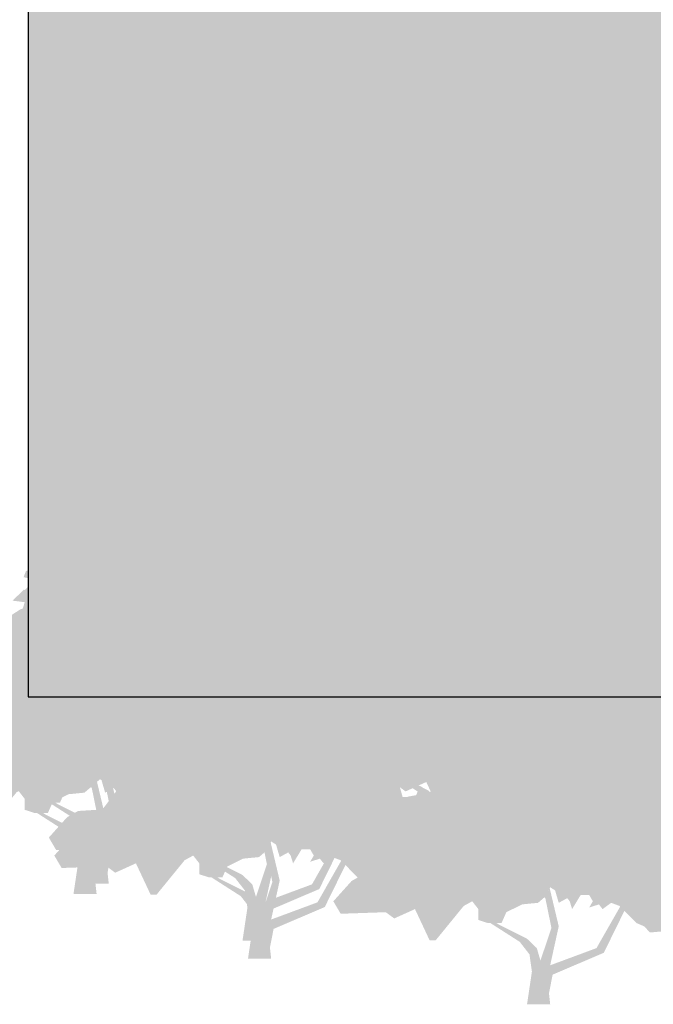
# Model space of a CAD drawing. Units: feet. Extents: x 2368 to 3224, y 836 to 1229.
# Tile 2 of 9: x 2395 to 2413, y 844 to 873. Entities that reach past the tile are written whole.
import ezdxf

# ---------------------------------------------------------------- set-up
doc = ezdxf.new("R2010")
doc.units = ezdxf.units.FT
for name, color, linetype, lineweight in [('A-ELEV', 7, 'Continuous', 25), ('A-ELEV-PATT', 8, 'Continuous', 13), ('L-PLNT', 3, 'Continuous', 13)]:
    doc.layers.add(name, color=color, linetype=linetype, lineweight=lineweight)

msp = doc.modelspace()

# ---------------------------------------------------------------- hatches: boundary and pattern name
at = {"layer": 'A-ELEV-PATT'}
h = msp.add_hatch(color=256, dxfattribs=at)
h.dxf.hatch_style = 1
h.paths.add_polyline_path([(2443.042, 973.51), (2394.909, 973.51), (2394.909, 853.51), (2443.042, 853.51)])
h.paths.add_polyline_path([(2422.205, 920.108), (2422.205, 905.784), (2416.403, 905.784), (2416.403, 920.108)], flags=16)
h.paths.add_polyline_path([(2449.299, 970.694), (2443.042, 973.51), (2443.042, 853.51), (2449.299, 853.51)])
h.paths.add_polyline_path([(2510.022, 987.861), (2368.302, 987.861), (2394.909, 973.51), (2443.042, 973.51), (2510.022, 973.51)])
h.paths.add_polyline_path([(2510.022, 973.51), (2443.042, 973.51), (2449.299, 970.694), (2510.022, 970.694)])
at = {"layer": 'L-PLNT'}
h = msp.add_hatch(color=256, dxfattribs=at)
h.dxf.hatch_style = 1
h.paths.add_polyline_path([(2411.665, 856.088), (2411.09, 856.687), (2410.371, 856.917), (2410.694, 857.424), (2410.407, 858.3), (2410.227, 858.3), (2409.868, 859.083), (2409.652, 859.037), (2409.4, 859.037), (2409.221, 859.406), (2409.328, 859.913), (2409.616, 859.913), (2409.077, 860.558), (2409.004, 861.069), (2408.717, 861.387), (2408.466, 861.111), (2408.322, 861.203), (2408.286, 861.433), (2408.106, 861.525), (2407.855, 861.295), (2407.567, 861.341), (2407.352, 860.926), (2407.352, 860.558), (2407.639, 860.419), (2407.423, 860.281), (2407.208, 860.466), (2406.597, 859.867), (2406.597, 859.728), (2406.345, 859.59), (2406.417, 859.452), (2406.597, 859.175), (2406.273, 858.945), (2405.95, 859.175), (2405.77, 859.129), (2405.698, 858.945), (2405.95, 858.899), (2405.986, 858.53), (2405.705, 858.576), (2405.375, 858.254), (2405.734, 858.208), (2405.59, 857.747), (2405.267, 857.701), (2404.907, 857.47), (2404.476, 857.24), (2404.44, 857.424), (2404.116, 856.733), (2404.692, 856.871), (2405.051, 856.641), (2404.943, 856.088), (2404.296, 855.857), (2404.009, 856.042), (2403.901, 855.765), (2403.649, 855.719), (2403.434, 855.443), (2403.182, 855.12), (2403.505, 854.844), (2403.721, 854.982), (2403.477, 854.581), (2403.654, 854.602), (2403.629, 854.239), (2403.038, 853.461), (2402.319, 853.415), (2401.996, 853.231), (2401.457, 852.632), (2401.672, 852.263), (2403.002, 852.309), (2403.254, 852.125), (2403.865, 852.401), (2404.296, 851.48), (2404.476, 851.48), (2405.303, 852.493), (2405.554, 852.632), (2405.734, 852.401), (2405.734, 852.079), (2406.022, 851.987), (2406.417, 851.987), (2406.561, 852.309), (2407.028, 852.54), (2407.495, 852.586), (2407.711, 852.77), (2407.747, 852.816), (2407.855, 853.046), (2407.999, 852.954), (2408.106, 852.586), (2408.358, 852.724), (2408.43, 852.632), (2408.502, 852.401), (2408.753, 852.816), (2409.005, 852.816), (2409.113, 852.632), (2409.005, 852.447), (2409.293, 852.54), (2409.4, 852.401), (2409.652, 852.586), (2409.904, 852.493), (2410.407, 851.987), (2410.622, 851.894), (2410.802, 851.71), (2412.312, 851.848), (2412.599, 851.572), (2412.815, 851.664), (2412.24, 852.401), (2412.204, 852.678), (2412.384, 852.954), (2412.06, 853.83), (2411.881, 853.83), (2411.521, 855.12), (2411.162, 855.166), (2411.377, 855.351)])
h = msp.add_hatch(color=256, dxfattribs=at)
h.dxf.hatch_style = 1
h.paths.add_polyline_path([(2411.214, 855.304), (2410.639, 855.904), (2409.92, 856.134), (2410.243, 856.641), (2409.956, 857.516), (2409.776, 857.516), (2409.417, 858.3), (2409.201, 858.254), (2408.949, 858.254), (2408.77, 858.622), (2408.878, 859.129), (2409.165, 859.129), (2408.626, 859.774), (2408.553, 860.286), (2408.266, 860.604), (2408.015, 860.327), (2407.871, 860.42), (2407.835, 860.65), (2407.655, 860.742), (2407.404, 860.512), (2407.116, 860.558), (2406.901, 860.143), (2406.901, 859.774), (2407.188, 859.636), (2406.972, 859.498), (2406.757, 859.682), (2406.146, 859.083), (2406.146, 858.945), (2405.894, 858.807), (2405.966, 858.668), (2406.146, 858.392), (2405.822, 858.162), (2405.499, 858.392), (2405.319, 858.346), (2405.247, 858.162), (2405.499, 858.115), (2405.535, 857.747), (2405.254, 857.793), (2404.924, 857.47), (2405.283, 857.424), (2405.139, 856.963), (2404.816, 856.917), (2404.456, 856.687), (2404.025, 856.456), (2403.989, 856.641), (2403.666, 855.95), (2404.241, 856.088), (2404.6, 855.857), (2404.492, 855.304), (2403.845, 855.074), (2403.558, 855.258), (2403.45, 854.982), (2403.198, 854.936), (2402.983, 854.659), (2402.731, 854.337), (2403.054, 854.06), (2403.27, 854.199), (2403.026, 853.798), (2403.203, 853.818), (2403.178, 853.456), (2402.587, 852.678), (2401.868, 852.632), (2401.545, 852.447), (2401.006, 851.848), (2401.221, 851.48), (2402.551, 851.526), (2402.803, 851.341), (2403.414, 851.618), (2403.845, 850.696), (2404.025, 850.696), (2404.852, 851.71), (2405.103, 851.848), (2405.283, 851.618), (2405.283, 851.295), (2405.571, 851.203), (2405.966, 851.203), (2406.11, 851.526), (2406.577, 851.756), (2407.044, 851.802), (2407.26, 851.987), (2407.296, 852.033), (2407.404, 852.263), (2407.548, 852.171), (2407.655, 851.802), (2407.907, 851.941), (2407.979, 851.848), (2408.051, 851.618), (2408.302, 852.033), (2408.554, 852.033), (2408.662, 851.848), (2408.554, 851.664), (2408.842, 851.756), (2408.949, 851.618), (2409.201, 851.802), (2409.453, 851.71), (2409.956, 851.203), (2410.172, 851.111), (2410.351, 850.927), (2411.861, 851.065), (2412.149, 850.788), (2412.364, 850.881), (2411.789, 851.618), (2411.753, 851.894), (2411.933, 852.171), (2411.609, 853.046), (2411.43, 853.046), (2411.07, 854.337), (2410.711, 854.383), (2410.926, 854.567)])
h = msp.add_hatch(color=256, dxfattribs=at)
h.dxf.hatch_style = 1
h.paths.add_polyline_path([(2414.456, 854.681), (2413.881, 855.281), (2413.162, 855.511), (2413.485, 856.018), (2413.198, 856.893), (2413.018, 856.893), (2412.659, 857.677), (2412.443, 857.631), (2412.191, 857.631), (2412.012, 857.999), (2412.12, 858.506), (2412.407, 858.506), (2411.868, 859.151), (2411.795, 859.663), (2411.509, 859.981), (2411.257, 859.704), (2411.113, 859.797), (2411.077, 860.027), (2410.897, 860.119), (2410.646, 859.889), (2410.358, 859.935), (2410.143, 859.52), (2410.143, 859.151), (2410.43, 859.013), (2410.214, 858.875), (2409.999, 859.059), (2409.388, 858.46), (2409.388, 858.322), (2409.136, 858.184), (2409.208, 858.045), (2409.388, 857.769), (2409.064, 857.539), (2408.741, 857.769), (2408.561, 857.723), (2408.489, 857.539), (2408.741, 857.492), (2408.777, 857.124), (2408.496, 857.17), (2408.166, 856.847), (2408.525, 856.801), (2408.381, 856.34), (2408.058, 856.294), (2407.698, 856.064), (2407.267, 855.834), (2407.231, 856.018), (2406.908, 855.327), (2407.483, 855.465), (2407.842, 855.234), (2407.734, 854.681), (2407.087, 854.451), (2406.8, 854.635), (2406.692, 854.359), (2406.44, 854.313), (2406.225, 854.036), (2405.973, 853.714), (2406.297, 853.437), (2406.512, 853.576), (2406.268, 853.175), (2406.445, 853.195), (2406.42, 852.833), (2405.829, 852.055), (2405.11, 852.009), (2404.787, 851.824), (2404.248, 851.225), (2404.463, 850.857), (2405.793, 850.903), (2406.045, 850.718), (2406.656, 850.995), (2407.087, 850.073), (2407.267, 850.073), (2408.094, 851.087), (2408.345, 851.225), (2408.525, 850.995), (2408.525, 850.672), (2408.813, 850.58), (2409.208, 850.58), (2409.352, 850.903), (2409.819, 851.133), (2410.286, 851.179), (2410.502, 851.364), (2410.538, 851.41), (2410.646, 851.64), (2410.79, 851.548), (2410.897, 851.179), (2411.149, 851.318), (2411.221, 851.225), (2411.293, 850.995), (2411.544, 851.41), (2411.796, 851.41), (2411.904, 851.225), (2411.796, 851.041), (2412.084, 851.133), (2412.191, 850.995), (2412.443, 851.179), (2412.695, 851.087), (2413.198, 850.58), (2413.414, 850.488), (2413.593, 850.304), (2415.103, 850.442), (2415.391, 850.165), (2415.606, 850.258), (2415.031, 850.995), (2414.995, 851.271), (2415.175, 851.548), (2414.851, 852.423), (2414.672, 852.423), (2414.312, 853.714), (2413.953, 853.76), (2414.168, 853.944)])
h = msp.add_hatch(color=256, dxfattribs=at)
h.dxf.hatch_style = 1
h.paths.add_polyline_path([(2421.127, 854.737), (2420.552, 855.336), (2419.833, 855.567), (2420.157, 856.074), (2419.869, 856.949), (2419.689, 856.949), (2419.33, 857.732), (2419.114, 857.686), (2418.862, 857.686), (2418.683, 858.055), (2418.791, 858.562), (2419.078, 858.562), (2418.539, 859.207), (2418.466, 859.718), (2418.18, 860.037), (2417.928, 859.76), (2417.784, 859.852), (2417.748, 860.083), (2417.568, 860.175), (2417.317, 859.944), (2417.029, 859.99), (2416.814, 859.576), (2416.814, 859.207), (2417.101, 859.069), (2416.886, 858.931), (2416.67, 859.115), (2416.059, 858.516), (2416.059, 858.378), (2415.807, 858.239), (2415.879, 858.101), (2416.059, 857.825), (2415.735, 857.594), (2415.412, 857.825), (2415.232, 857.779), (2415.16, 857.594), (2415.412, 857.548), (2415.448, 857.179), (2415.167, 857.226), (2414.837, 856.903), (2415.196, 856.857), (2415.052, 856.396), (2414.729, 856.35), (2414.369, 856.12), (2413.938, 855.889), (2413.902, 856.074), (2413.579, 855.382), (2414.154, 855.521), (2414.513, 855.29), (2414.405, 854.737), (2413.758, 854.507), (2413.471, 854.691), (2413.363, 854.415), (2413.111, 854.369), (2412.896, 854.092), (2412.644, 853.769), (2412.968, 853.493), (2413.183, 853.631), (2412.939, 853.23), (2413.117, 853.251), (2413.091, 852.888), (2412.5, 852.111), (2411.781, 852.064), (2411.458, 851.88), (2410.919, 851.281), (2411.134, 850.912), (2412.464, 850.958), (2412.716, 850.774), (2413.327, 851.051), (2413.758, 850.129), (2413.938, 850.129), (2414.765, 851.143), (2415.016, 851.281), (2415.196, 851.051), (2415.196, 850.728), (2415.484, 850.636), (2415.879, 850.636), (2416.023, 850.958), (2416.49, 851.189), (2416.957, 851.235), (2417.173, 851.419), (2417.209, 851.465), (2417.317, 851.696), (2417.461, 851.604), (2417.568, 851.235), (2417.82, 851.373), (2417.892, 851.281), (2417.964, 851.051), (2418.215, 851.465), (2418.467, 851.465), (2418.575, 851.281), (2418.467, 851.097), (2418.755, 851.189), (2418.862, 851.051), (2419.114, 851.235), (2419.366, 851.143), (2419.869, 850.636), (2420.085, 850.544), (2420.264, 850.359), (2421.774, 850.498), (2422.062, 850.221), (2422.277, 850.313), (2421.702, 851.051), (2421.666, 851.327), (2421.846, 851.604), (2421.522, 852.479), (2421.343, 852.479), (2420.983, 853.769), (2420.624, 853.816), (2420.839, 854)])
h = msp.add_hatch(color=256, dxfattribs=at)
h.dxf.hatch_style = 1
h.paths.add_polyline_path([(2401.097, 854.492), (2400.522, 855.091), (2399.803, 855.321), (2400.126, 855.828), (2399.839, 856.704), (2399.659, 856.704), (2399.3, 857.487), (2399.084, 857.441), (2398.832, 857.441), (2398.653, 857.809), (2398.76, 858.316), (2399.048, 858.316), (2398.509, 858.962), (2398.436, 859.473), (2398.149, 859.791), (2397.898, 859.514), (2397.754, 859.607), (2397.718, 859.837), (2397.538, 859.929), (2397.287, 859.699), (2396.999, 859.745), (2396.783, 859.33), (2396.783, 858.962), (2397.071, 858.823), (2396.855, 858.685), (2396.64, 858.869), (2396.029, 858.27), (2396.029, 858.132), (2395.777, 857.994), (2395.849, 857.856), (2396.029, 857.579), (2395.705, 857.349), (2395.382, 857.579), (2395.202, 857.533), (2395.13, 857.349), (2395.382, 857.303), (2395.418, 856.934), (2395.136, 856.98), (2394.806, 856.657), (2395.166, 856.611), (2395.022, 856.151), (2394.699, 856.104), (2394.339, 855.874), (2393.908, 855.644), (2393.872, 855.828), (2393.548, 855.137), (2394.124, 855.275), (2394.483, 855.045), (2394.375, 854.492), (2393.728, 854.261), (2393.441, 854.446), (2393.333, 854.169), (2393.081, 854.123), (2392.865, 853.846), (2392.614, 853.524), (2392.937, 853.247), (2393.153, 853.386), (2392.909, 852.985), (2393.086, 853.006), (2393.061, 852.643), (2392.47, 851.865), (2391.751, 851.819), (2391.428, 851.635), (2390.888, 851.035), (2391.104, 850.667), (2392.434, 850.713), (2392.686, 850.529), (2393.297, 850.805), (2393.728, 849.883), (2393.908, 849.883), (2394.735, 850.897), (2394.986, 851.035), (2395.166, 850.805), (2395.166, 850.483), (2395.453, 850.39), (2395.849, 850.39), (2395.993, 850.713), (2396.46, 850.943), (2396.927, 850.989), (2397.143, 851.174), (2397.179, 851.22), (2397.287, 851.45), (2397.43, 851.358), (2397.538, 850.989), (2397.79, 851.128), (2397.862, 851.035), (2397.934, 850.805), (2398.185, 851.22), (2398.437, 851.22), (2398.545, 851.035), (2398.437, 850.851), (2398.724, 850.943), (2398.832, 850.805), (2399.084, 850.989), (2399.336, 850.897), (2399.839, 850.39), (2400.054, 850.298), (2400.234, 850.114), (2401.744, 850.252), (2402.031, 849.976), (2402.247, 850.068), (2401.672, 850.805), (2401.636, 851.082), (2401.816, 851.358), (2401.492, 852.234), (2401.312, 852.234), (2400.953, 853.524), (2400.594, 853.57), (2400.809, 853.754)])
h = msp.add_hatch(color=256, dxfattribs=at)
h.dxf.hatch_style = 1
h.paths.add_polyline_path([(2400.74, 854.183), (2400.164, 854.782), (2399.446, 855.013), (2399.769, 855.519), (2399.482, 856.395), (2399.302, 856.395), (2398.942, 857.178), (2398.727, 857.132), (2398.475, 857.132), (2398.295, 857.501), (2398.403, 858.008), (2398.691, 858.008), (2398.152, 858.653), (2398.079, 859.164), (2397.792, 859.482), (2397.54, 859.206), (2397.397, 859.298), (2397.361, 859.529), (2397.181, 859.621), (2396.929, 859.39), (2396.642, 859.436), (2396.426, 859.022), (2396.426, 858.653), (2396.714, 858.515), (2396.498, 858.377), (2396.282, 858.561), (2395.671, 857.962), (2395.671, 857.824), (2395.42, 857.685), (2395.492, 857.547), (2395.671, 857.271), (2395.348, 857.04), (2395.024, 857.271), (2394.845, 857.224), (2394.773, 857.04), (2395.024, 856.994), (2395.06, 856.625), (2394.779, 856.672), (2394.449, 856.349), (2394.809, 856.303), (2394.665, 855.842), (2394.341, 855.796), (2393.982, 855.566), (2393.551, 855.335), (2393.515, 855.519), (2393.191, 854.828), (2393.766, 854.966), (2394.126, 854.736), (2394.018, 854.183), (2393.371, 853.953), (2393.083, 854.137), (2392.975, 853.861), (2392.724, 853.814), (2392.508, 853.538), (2392.257, 853.215), (2392.58, 852.939), (2392.796, 853.077), (2392.552, 852.676), (2392.729, 852.697), (2392.703, 852.334), (2392.113, 851.556), (2391.394, 851.51), (2391.07, 851.326), (2390.531, 850.727), (2390.747, 850.358), (2392.077, 850.404), (2392.328, 850.22), (2392.94, 850.497), (2393.371, 849.575), (2393.551, 849.575), (2394.377, 850.589), (2394.629, 850.727), (2394.809, 850.497), (2394.809, 850.174), (2395.096, 850.082), (2395.492, 850.082), (2395.635, 850.404), (2396.103, 850.635), (2396.57, 850.681), (2396.786, 850.865), (2396.822, 850.911), (2396.929, 851.142), (2397.073, 851.05), (2397.181, 850.681), (2397.433, 850.819), (2397.505, 850.727), (2397.576, 850.497), (2397.828, 850.911), (2398.08, 850.911), (2398.187, 850.727), (2398.08, 850.543), (2398.367, 850.635), (2398.475, 850.497), (2398.727, 850.681), (2398.978, 850.589), (2399.482, 850.082), (2399.697, 849.99), (2399.877, 849.805), (2401.387, 849.944), (2401.674, 849.667), (2401.89, 849.759), (2401.315, 850.497), (2401.279, 850.773), (2401.458, 851.05), (2401.135, 851.925), (2400.955, 851.925), (2400.596, 853.215), (2400.236, 853.261), (2400.452, 853.446)])
h = msp.add_hatch(color=256, dxfattribs=at)
h.dxf.hatch_style = 1
h.paths.add_polyline_path([(2422.561, 854.308), (2421.986, 854.907), (2421.267, 855.137), (2421.591, 855.644), (2421.303, 856.52), (2421.123, 856.52), (2420.764, 857.303), (2420.548, 857.257), (2420.297, 857.257), (2420.117, 857.626), (2420.225, 858.132), (2420.512, 858.132), (2419.973, 858.778), (2419.901, 859.289), (2419.614, 859.607), (2419.362, 859.331), (2419.218, 859.423), (2419.182, 859.653), (2419.003, 859.745), (2418.751, 859.515), (2418.463, 859.561), (2418.248, 859.146), (2418.248, 858.778), (2418.535, 858.639), (2418.32, 858.501), (2418.104, 858.685), (2417.493, 858.086), (2417.493, 857.948), (2417.241, 857.81), (2417.313, 857.672), (2417.493, 857.395), (2417.169, 857.165), (2416.846, 857.395), (2416.666, 857.349), (2416.594, 857.165), (2416.846, 857.119), (2416.882, 856.75), (2416.601, 856.796), (2416.271, 856.474), (2416.63, 856.427), (2416.486, 855.967), (2416.163, 855.921), (2415.804, 855.69), (2415.372, 855.46), (2415.336, 855.644), (2415.013, 854.953), (2415.588, 855.091), (2415.947, 854.861), (2415.839, 854.308), (2415.192, 854.077), (2414.905, 854.262), (2414.797, 853.985), (2414.545, 853.939), (2414.33, 853.663), (2414.078, 853.34), (2414.402, 853.063), (2414.617, 853.202), (2414.374, 852.801), (2414.551, 852.822), (2414.525, 852.459), (2413.934, 851.681), (2413.215, 851.635), (2412.892, 851.451), (2412.353, 850.852), (2412.568, 850.483), (2413.898, 850.529), (2414.15, 850.345), (2414.761, 850.621), (2415.192, 849.7), (2415.372, 849.7), (2416.199, 850.713), (2416.451, 850.852), (2416.63, 850.621), (2416.63, 850.299), (2416.918, 850.206), (2417.313, 850.206), (2417.457, 850.529), (2417.924, 850.759), (2418.392, 850.806), (2418.607, 850.99), (2418.643, 851.036), (2418.751, 851.266), (2418.895, 851.174), (2419.003, 850.806), (2419.254, 850.944), (2419.326, 850.852), (2419.398, 850.621), (2419.65, 851.036), (2419.901, 851.036), (2420.009, 850.852), (2419.901, 850.667), (2420.189, 850.759), (2420.297, 850.621), (2420.548, 850.806), (2420.8, 850.713), (2421.303, 850.206), (2421.519, 850.114), (2421.698, 849.93), (2423.208, 850.068), (2423.496, 849.792), (2423.711, 849.884), (2423.136, 850.621), (2423.1, 850.898), (2423.28, 851.174), (2422.957, 852.05), (2422.777, 852.05), (2422.417, 853.34), (2422.058, 853.386), (2422.274, 853.57)])
h = msp.add_hatch(color=256, dxfattribs=at)
h.dxf.hatch_style = 1
h.paths.add_polyline_path([(2405.727, 852.813), (2405.152, 853.412), (2404.433, 853.642), (2404.757, 854.149), (2404.469, 855.024), (2404.29, 855.024), (2403.93, 855.808), (2403.714, 855.762), (2403.463, 855.762), (2403.283, 856.13), (2403.391, 856.637), (2403.679, 856.637), (2403.139, 857.282), (2403.067, 857.794), (2402.78, 858.112), (2402.528, 857.835), (2402.384, 857.928), (2402.349, 858.158), (2402.169, 858.25), (2401.917, 858.02), (2401.63, 858.066), (2401.414, 857.651), (2401.414, 857.282), (2401.702, 857.144), (2401.486, 857.006), (2401.27, 857.19), (2400.659, 856.591), (2400.659, 856.453), (2400.408, 856.315), (2400.479, 856.177), (2400.659, 855.9), (2400.336, 855.67), (2400.012, 855.9), (2399.832, 855.854), (2399.761, 855.67), (2400.012, 855.624), (2400.048, 855.255), (2399.767, 855.301), (2399.437, 854.978), (2399.796, 854.932), (2399.653, 854.471), (2399.329, 854.425), (2398.97, 854.195), (2398.538, 853.965), (2398.502, 854.149), (2398.179, 853.458), (2398.754, 853.596), (2399.114, 853.366), (2399.006, 852.813), (2398.359, 852.582), (2398.071, 852.766), (2397.963, 852.49), (2397.712, 852.444), (2397.496, 852.167), (2397.244, 851.845), (2397.568, 851.568), (2397.784, 851.707), (2397.54, 851.306), (2397.717, 851.327), (2397.691, 850.964), (2397.101, 850.186), (2396.382, 850.14), (2396.058, 849.956), (2395.519, 849.356), (2395.735, 848.988), (2397.065, 849.034), (2397.316, 848.85), (2397.927, 849.126), (2398.359, 848.204), (2398.538, 848.204), (2399.365, 849.218), (2399.617, 849.356), (2399.796, 849.126), (2399.796, 848.803), (2400.084, 848.711), (2400.479, 848.711), (2400.623, 849.034), (2401.09, 849.264), (2401.558, 849.31), (2401.773, 849.495), (2401.809, 849.541), (2401.917, 849.771), (2402.061, 849.679), (2402.169, 849.31), (2402.42, 849.449), (2402.492, 849.356), (2402.564, 849.126), (2402.816, 849.541), (2403.067, 849.541), (2403.175, 849.356), (2403.067, 849.172), (2403.355, 849.264), (2403.463, 849.126), (2403.714, 849.31), (2403.966, 849.218), (2404.469, 848.711), (2404.685, 848.619), (2404.865, 848.435), (2406.374, 848.573), (2406.662, 848.297), (2406.878, 848.389), (2406.302, 849.126), (2406.267, 849.403), (2406.446, 849.679), (2406.123, 850.555), (2405.943, 850.555), (2405.584, 851.845), (2405.224, 851.891), (2405.44, 852.075)])
h = msp.add_hatch(color=256, dxfattribs=at)
h.dxf.hatch_style = 1
h.paths.add_polyline_path([(2405.889, 852.281), (2405.314, 852.88), (2404.595, 853.111), (2404.919, 853.618), (2404.631, 854.493), (2404.452, 854.493), (2404.092, 855.277), (2403.876, 855.231), (2403.625, 855.231), (2403.445, 855.599), (2403.553, 856.106), (2403.84, 856.106), (2403.301, 856.751), (2403.229, 857.263), (2402.942, 857.581), (2402.69, 857.304), (2402.546, 857.396), (2402.51, 857.627), (2402.331, 857.719), (2402.079, 857.489), (2401.792, 857.535), (2401.576, 857.12), (2401.576, 856.751), (2401.863, 856.613), (2401.648, 856.475), (2401.432, 856.659), (2400.821, 856.06), (2400.821, 855.922), (2400.569, 855.784), (2400.641, 855.645), (2400.821, 855.369), (2400.498, 855.138), (2400.174, 855.369), (2399.994, 855.323), (2399.922, 855.138), (2400.174, 855.092), (2400.21, 854.724), (2399.929, 854.77), (2399.599, 854.447), (2399.958, 854.401), (2399.815, 853.94), (2399.491, 853.894), (2399.132, 853.664), (2398.7, 853.433), (2398.664, 853.618), (2398.341, 852.927), (2398.916, 853.065), (2399.275, 852.834), (2399.168, 852.281), (2398.521, 852.051), (2398.233, 852.235), (2398.125, 851.959), (2397.874, 851.913), (2397.658, 851.636), (2397.406, 851.314), (2397.73, 851.037), (2397.946, 851.175), (2397.702, 850.775), (2397.879, 850.795), (2397.853, 850.433), (2397.263, 849.655), (2396.544, 849.609), (2396.22, 849.424), (2395.681, 848.825), (2395.897, 848.457), (2397.227, 848.503), (2397.478, 848.318), (2398.089, 848.595), (2398.521, 847.673), (2398.7, 847.673), (2399.527, 848.687), (2399.779, 848.825), (2399.958, 848.595), (2399.958, 848.272), (2400.246, 848.18), (2400.641, 848.18), (2400.785, 848.503), (2401.252, 848.733), (2401.72, 848.779), (2401.935, 848.964), (2401.971, 849.01), (2402.079, 849.24), (2402.223, 849.148), (2402.331, 848.779), (2402.582, 848.917), (2402.654, 848.825), (2402.726, 848.595), (2402.978, 849.01), (2403.229, 849.01), (2403.337, 848.825), (2403.229, 848.641), (2403.517, 848.733), (2403.625, 848.595), (2403.876, 848.779), (2404.128, 848.687), (2404.631, 848.18), (2404.847, 848.088), (2405.027, 847.904), (2406.536, 848.042), (2406.824, 847.765), (2407.04, 847.858), (2406.464, 848.595), (2406.428, 848.871), (2406.608, 849.148), (2406.285, 850.023), (2406.105, 850.023), (2405.746, 851.314), (2405.386, 851.36), (2405.602, 851.544)])
h = msp.add_hatch(color=256, dxfattribs=at)
h.dxf.hatch_style = 1
h.paths.add_polyline_path([(2419.444, 852.439), (2418.869, 853.038), (2418.15, 853.268), (2418.473, 853.775), (2418.186, 854.651), (2418.006, 854.651), (2417.647, 855.434), (2417.431, 855.388), (2417.179, 855.388), (2417, 855.757), (2417.107, 856.264), (2417.395, 856.264), (2416.856, 856.909), (2416.783, 857.42), (2416.496, 857.738), (2416.245, 857.462), (2416.101, 857.554), (2416.065, 857.784), (2415.885, 857.876), (2415.634, 857.646), (2415.346, 857.692), (2415.13, 857.277), (2415.13, 856.909), (2415.418, 856.77), (2415.202, 856.632), (2414.987, 856.817), (2414.376, 856.217), (2414.376, 856.079), (2414.124, 855.941), (2414.196, 855.803), (2414.376, 855.526), (2414.052, 855.296), (2413.729, 855.526), (2413.549, 855.48), (2413.477, 855.296), (2413.729, 855.25), (2413.764, 854.881), (2413.483, 854.927), (2413.153, 854.605), (2413.513, 854.559), (2413.369, 854.098), (2413.046, 854.052), (2412.686, 853.821), (2412.255, 853.591), (2412.219, 853.775), (2411.895, 853.084), (2412.47, 853.222), (2412.83, 852.992), (2412.722, 852.439), (2412.075, 852.208), (2411.788, 852.393), (2411.68, 852.116), (2411.428, 852.07), (2411.212, 851.794), (2410.961, 851.471), (2411.284, 851.195), (2411.5, 851.333), (2411.256, 850.932), (2411.433, 850.953), (2411.408, 850.59), (2410.817, 849.812), (2410.098, 849.766), (2409.775, 849.582), (2409.235, 848.983), (2409.451, 848.614), (2410.781, 848.66), (2411.033, 848.476), (2411.644, 848.752), (2412.075, 847.831), (2412.255, 847.831), (2413.082, 848.844), (2413.333, 848.983), (2413.513, 848.752), (2413.513, 848.43), (2413.8, 848.338), (2414.196, 848.338), (2414.34, 848.66), (2414.807, 848.89), (2415.274, 848.937), (2415.49, 849.121), (2415.526, 849.167), (2415.634, 849.397), (2415.777, 849.305), (2415.885, 848.937), (2416.137, 849.075), (2416.209, 848.983), (2416.281, 848.752), (2416.532, 849.167), (2416.784, 849.167), (2416.892, 848.983), (2416.784, 848.798), (2417.071, 848.89), (2417.179, 848.752), (2417.431, 848.937), (2417.682, 848.844), (2418.186, 848.338), (2418.401, 848.245), (2418.581, 848.061), (2420.091, 848.199), (2420.378, 847.923), (2420.594, 848.015), (2420.019, 848.752), (2419.983, 849.029), (2420.163, 849.305), (2419.839, 850.181), (2419.659, 850.181), (2419.3, 851.471), (2418.941, 851.517), (2419.156, 851.701)])
h = msp.add_hatch(color=256, dxfattribs=at)
h.dxf.hatch_style = 1
h.paths.add_polyline_path([(2414.123, 850.931), (2413.547, 851.53), (2412.829, 851.76), (2413.152, 852.267), (2412.865, 853.143), (2412.685, 853.143), (2412.325, 853.926), (2412.11, 853.88), (2411.858, 853.88), (2411.678, 854.249), (2411.786, 854.756), (2412.074, 854.756), (2411.535, 855.401), (2411.462, 855.912), (2411.175, 856.23), (2410.924, 855.954), (2410.78, 856.046), (2410.744, 856.276), (2410.564, 856.368), (2410.312, 856.138), (2410.025, 856.184), (2409.809, 855.769), (2409.809, 855.401), (2410.097, 855.262), (2409.881, 855.124), (2409.665, 855.309), (2409.054, 854.709), (2409.054, 854.571), (2408.803, 854.433), (2408.875, 854.295), (2409.054, 854.018), (2408.731, 853.788), (2408.407, 854.018), (2408.228, 853.972), (2408.156, 853.788), (2408.407, 853.742), (2408.443, 853.373), (2408.162, 853.419), (2407.832, 853.097), (2408.192, 853.051), (2408.048, 852.59), (2407.724, 852.544), (2407.365, 852.313), (2406.934, 852.083), (2406.898, 852.267), (2406.574, 851.576), (2407.149, 851.714), (2407.509, 851.484), (2407.401, 850.931), (2406.754, 850.7), (2406.466, 850.885), (2406.359, 850.608), (2406.107, 850.562), (2405.891, 850.286), (2405.64, 849.963), (2405.963, 849.687), (2406.179, 849.825), (2405.935, 849.424), (2406.112, 849.445), (2406.086, 849.082), (2405.496, 848.304), (2404.777, 848.258), (2404.453, 848.074), (2403.914, 847.475), (2404.13, 847.106), (2405.46, 847.152), (2405.711, 846.968), (2406.323, 847.244), (2406.754, 846.323), (2406.934, 846.323), (2407.76, 847.336), (2408.012, 847.475), (2408.192, 847.244), (2408.192, 846.922), (2408.479, 846.83), (2408.875, 846.83), (2409.018, 847.152), (2409.486, 847.383), (2409.953, 847.429), (2410.169, 847.613), (2410.205, 847.659), (2410.312, 847.889), (2410.456, 847.797), (2410.564, 847.429), (2410.816, 847.567), (2410.888, 847.475), (2410.959, 847.244), (2411.211, 847.659), (2411.463, 847.659), (2411.571, 847.475), (2411.463, 847.29), (2411.75, 847.383), (2411.858, 847.244), (2412.11, 847.429), (2412.361, 847.336), (2412.865, 846.83), (2413.08, 846.737), (2413.26, 846.553), (2414.77, 846.691), (2415.057, 846.415), (2415.273, 846.507), (2414.698, 847.244), (2414.662, 847.521), (2414.841, 847.797), (2414.518, 848.673), (2414.338, 848.673), (2413.979, 849.963), (2413.619, 850.009), (2413.835, 850.193)])
h = msp.add_hatch(color=256, dxfattribs=at)
h.dxf.hatch_style = 1
h.paths.add_polyline_path([(2407.927, 850.466), (2409.436, 851.111), (2410.045, 852.351), (2409.92, 852.477), (2409.904, 852.447), (2409.221, 851.249), (2407.855, 850.742), (2408.106, 851.894), (2407.855, 852.954), (2407.84, 853.015), (2407.747, 852.816), (2407.711, 852.77), (2407.688, 852.751), (2407.711, 852.724), (2407.891, 851.848), (2407.567, 850.881), (2407.459, 851.249), (2407.172, 851.526), (2406.345, 851.94), (2406.274, 851.987), (2406.093, 851.987), (2406.956, 851.434), (2407.244, 851.065), (2407.316, 850.558), (2407.172, 849.59), (2407.855, 849.59), (2407.819, 849.913)])
h = msp.add_hatch(color=256, dxfattribs=at)
h.dxf.hatch_style = 1
h.paths.add_polyline_path([(2407.476, 849.683), (2408.985, 850.328), (2409.594, 851.567), (2409.469, 851.693), (2409.453, 851.664), (2408.77, 850.466), (2407.404, 849.959), (2407.655, 851.111), (2407.404, 852.171), (2407.389, 852.232), (2407.296, 852.033), (2407.26, 851.987), (2407.237, 851.967), (2407.26, 851.941), (2407.44, 851.065), (2407.116, 850.097), (2407.008, 850.466), (2406.721, 850.742), (2405.894, 851.157), (2405.823, 851.203), (2405.642, 851.203), (2406.505, 850.65), (2406.793, 850.282), (2406.865, 849.775), (2406.721, 848.807), (2407.404, 848.807), (2407.368, 849.13)])
h = msp.add_hatch(color=256, dxfattribs=at)
h.dxf.hatch_style = 1
h.paths.add_polyline_path([(2397.359, 848.87), (2398.868, 849.515), (2399.477, 850.755), (2399.352, 850.88), (2399.336, 850.851), (2398.653, 849.653), (2397.287, 849.146), (2397.538, 850.298), (2397.287, 851.358), (2397.272, 851.419), (2397.179, 851.22), (2397.143, 851.174), (2397.12, 851.154), (2397.143, 851.128), (2397.323, 850.252), (2396.999, 849.284), (2396.891, 849.653), (2396.604, 849.93), (2395.777, 850.344), (2395.706, 850.39), (2395.525, 850.39), (2396.388, 849.837), (2396.676, 849.469), (2396.747, 848.962), (2396.604, 847.994), (2397.287, 847.994), (2397.251, 848.317)])
h = msp.add_hatch(color=256, dxfattribs=at)
h.dxf.hatch_style = 1
h.paths.add_polyline_path([(2410.718, 849.06), (2412.227, 849.705), (2412.836, 850.944), (2412.711, 851.07), (2412.695, 851.041), (2412.012, 849.843), (2410.646, 849.336), (2410.897, 850.488), (2410.646, 851.548), (2410.631, 851.609), (2410.538, 851.41), (2410.502, 851.364), (2410.479, 851.344), (2410.502, 851.318), (2410.682, 850.442), (2410.358, 849.474), (2410.25, 849.843), (2409.963, 850.119), (2409.136, 850.534), (2409.065, 850.58), (2408.885, 850.58), (2409.747, 850.027), (2410.035, 849.659), (2410.107, 849.152), (2409.963, 848.184), (2410.646, 848.184), (2410.61, 848.507)])
h = msp.add_hatch(color=256, dxfattribs=at)
h.dxf.hatch_style = 1
h.paths.add_polyline_path([(2397.001, 848.561), (2398.511, 849.206), (2399.12, 850.446), (2398.995, 850.572), (2398.978, 850.543), (2398.295, 849.345), (2396.929, 848.838), (2397.181, 849.99), (2396.929, 851.05), (2396.915, 851.111), (2396.822, 850.911), (2396.786, 850.865), (2396.763, 850.846), (2396.786, 850.819), (2396.965, 849.944), (2396.642, 848.976), (2396.534, 849.345), (2396.246, 849.621), (2395.42, 850.036), (2395.349, 850.082), (2395.168, 850.082), (2396.031, 849.529), (2396.318, 849.16), (2396.39, 848.653), (2396.246, 847.686), (2396.929, 847.686), (2396.893, 848.008)])
h = msp.add_hatch(color=256, dxfattribs=at)
h.dxf.hatch_style = 1
h.paths.add_polyline_path([(2401.989, 847.191), (2403.499, 847.836), (2404.108, 849.076), (2403.983, 849.201), (2403.966, 849.172), (2403.283, 847.974), (2401.917, 847.467), (2402.169, 848.619), (2401.917, 849.679), (2401.903, 849.74), (2401.809, 849.541), (2401.773, 849.495), (2401.751, 849.475), (2401.773, 849.449), (2401.953, 848.573), (2401.63, 847.605), (2401.522, 847.974), (2401.234, 848.25), (2400.408, 848.665), (2400.337, 848.711), (2400.156, 848.711), (2401.019, 848.158), (2401.306, 847.79), (2401.378, 847.283), (2401.234, 846.315), (2401.917, 846.315), (2401.881, 846.638)])
h = msp.add_hatch(color=256, dxfattribs=at)
h.dxf.hatch_style = 1
h.paths.add_polyline_path([(2402.151, 846.659), (2403.661, 847.305), (2404.27, 848.544), (2404.145, 848.67), (2404.128, 848.641), (2403.445, 847.443), (2402.079, 846.936), (2402.331, 848.088), (2402.079, 849.148), (2402.065, 849.209), (2401.971, 849.01), (2401.935, 848.964), (2401.913, 848.944), (2401.935, 848.917), (2402.115, 848.042), (2401.792, 847.074), (2401.684, 847.443), (2401.396, 847.719), (2400.569, 848.134), (2400.499, 848.18), (2400.318, 848.18), (2401.181, 847.627), (2401.468, 847.259), (2401.54, 846.752), (2401.396, 845.784), (2402.079, 845.784), (2402.043, 846.107)])
h = msp.add_hatch(color=256, dxfattribs=at)
h.dxf.hatch_style = 1
h.paths.add_polyline_path([(2410.384, 845.309), (2411.894, 845.954), (2412.503, 847.194), (2412.378, 847.32), (2412.361, 847.29), (2411.678, 846.092), (2410.312, 845.585), (2410.564, 846.737), (2410.312, 847.797), (2410.298, 847.858), (2410.205, 847.659), (2410.169, 847.613), (2410.146, 847.593), (2410.169, 847.567), (2410.348, 846.691), (2410.025, 845.724), (2409.917, 846.092), (2409.629, 846.369), (2408.803, 846.783), (2408.732, 846.83), (2408.551, 846.83), (2409.414, 846.277), (2409.701, 845.908), (2409.773, 845.401), (2409.629, 844.433), (2410.312, 844.433), (2410.276, 844.756)])

# ---------------------------------------------------------------- linework, layer by layer
at = {"layer": 'A-ELEV'}
msp.add_line((2394.909, 853.51), (2521.044, 853.51), dxfattribs=at)
msp.add_line((2394.909, 853.51), (2521.044, 853.51), dxfattribs=at)
msp.add_lwpolyline([(2394.909, 853.51), (2443.042, 853.51), (2443.042, 973.51), (2394.909, 973.51)], close=True, dxfattribs=at)
msp.add_lwpolyline([(2394.909, 853.51), (2443.042, 853.51), (2443.042, 973.51), (2394.909, 973.51)], close=True, dxfattribs=at)

doc.saveas('drawing.dxf')
